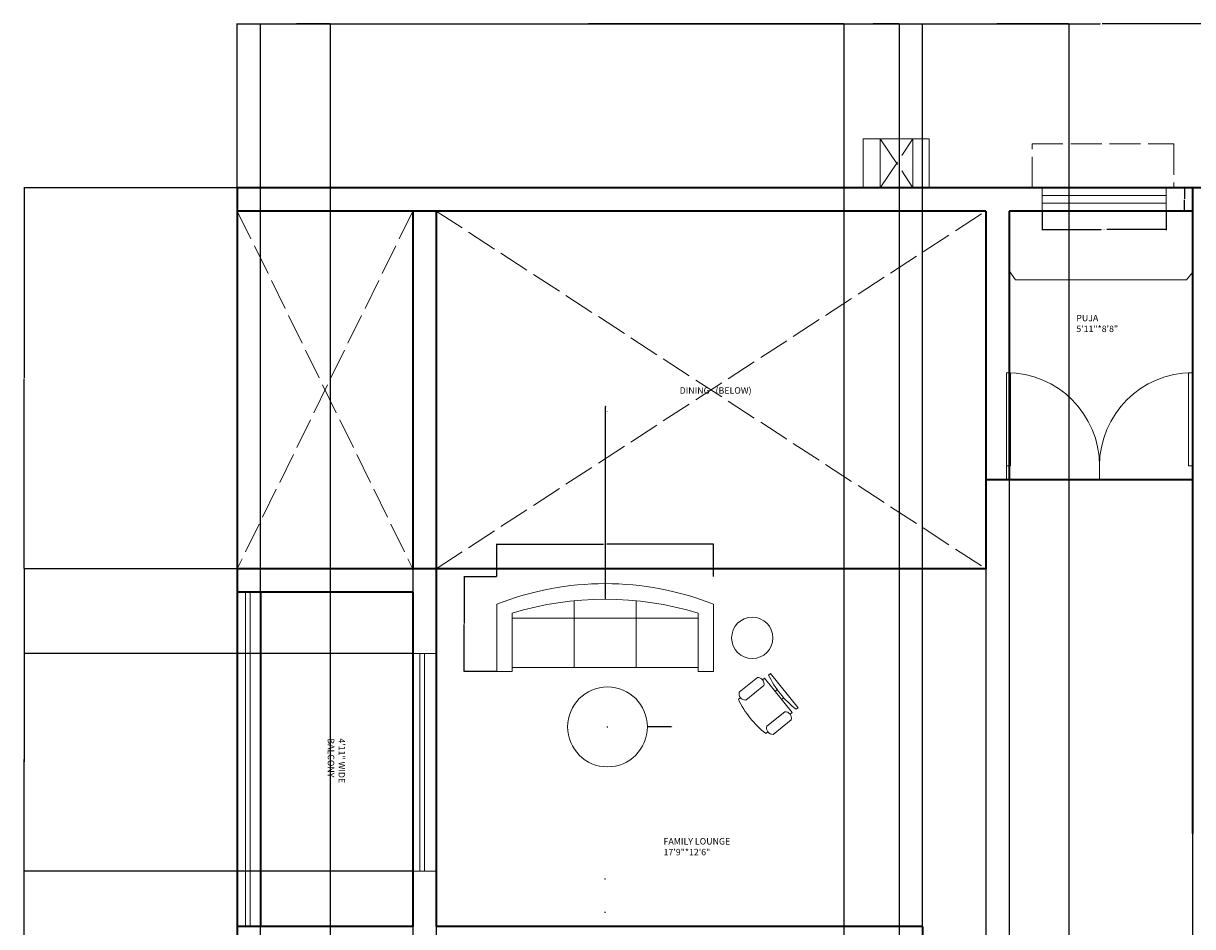
# Model space of a CAD drawing. Units: inches. Extents: x 293720 to 590083, y 155482 to 312405.
# Tile 3 of 4: x 293720 to 294173, y 156028 to 156378. Entities that reach past the tile are written whole.
import ezdxf

# ---------------------------------------------------------------- set-up
doc = ezdxf.new("R2010")
doc.units = ezdxf.units.IN
doc.linetypes.add('ACAD_ISO02W100', pattern=[15, 12, -3])
for name, color, linetype, lineweight in [('A-ANNO-DIMS', 2, 'Continuous', 18), ('A-AREA-IDEN', 7, 'Continuous', 18), ('A-DOOR', 3, 'Continuous', 18), ('A-FLOR-CASE', 8, 'Continuous', 18), ('A-FLOR-HRAL', 4, 'Continuous', 18), ('A-FLOR-OPEN', 8, 'ACAD_ISO02W100', 13), ('A-FLOR-OVHD', 8, 'ACAD_ISO02W100', 13), ('A-FLOR-PROJ', 8, 'Continuous', 18), ('A-FURN', 8, 'Continuous', 18), ('A-GLAZ', 4, 'Continuous', 18), ('A-WALL', 7, 'Continuous', 35)]:
    doc.layers.add(name, color=color, linetype=linetype, lineweight=lineweight)
doc.styles.get("Standard").update_dxf_attribs({"font": 'arial.ttf'})
doc.dimstyles.get("Standard").update_dxf_attribs({"dimtxt": 0.18, "dimasz": 0.18, "dimexe": 0.18, "dimexo": 0.0625, "dimgap": 0.09, "dimtad": 0, "dimtih": 1, "dimtoh": 1, "dimdec": 4, "dimzin": 0, "dimdsep": 46, "dimtxsty": 'Standard', "dimcen": 0.09, "dimadec": 0, "dimazin": 0, "dimtfac": 1, "dimtdec": 4, "dimtofl": 0, "dimtmove": 0, "dimatfit": 3, "dimfxl": 1, "dimtolj": 1, "dimtzin": 0, "dimarcsym": 0})

# ---------------------------------------------------------------- blocks, each defined once
blk = doc.blocks.new('Sofa - Roundback 7 ft.')
for p, q in [((-12.00002, -32.4421), (-12.00003, -6.5971)), ((11.99997, -32.4421), (11.99998, -6.5971)), ((-36.000027, -34), (-36.000027, -11.4696)), ((-35.999844, -13.3819), (35.9998, -13.3819)), ((35.99998, -34), (35.99998, -11.4696)), ((-36.000027, -32.4421), (35.99998, -32.4421))]:
    blk.add_line(p, q)
for points in [[(-36.000027, -34), (-42.000027, -34), (-42.000027, -8)], [(41.99998, -8), (41.99998, -34), (35.99998, -34)]]:
    blk.add_lwpolyline(points)
for centre, radius, start, end in [((0, -114.25), 114.25, 68.43141, 111.5686), ((-0.00001, -127.1968), 121.1968, 72.72033, 107.2797)]:
    blk.add_arc(centre, radius, start, end)
blk = doc.blocks.new('Chair - Desk')
for p, q in [((-8.5, 0), (-8.5, -1)), ((-8.5, 0), (8.5, 0)), ((8.5, 0), (8.5, -1)), ((-8.5, -3), (-8.5, -4)), ((-8.5, -3), (8.5, -3)), ((-2, -3), (-2, -1.9355)), ((2, -1.9576), (2, -3)), ((8.5, -3), (8.5, -4)), ((-10.5, -5), (-10.5, -14)), ((-6.5, -14), (-6.5, -5)), ((6.5, -5), (6.5, -14)), ((10.5, -14), (10.5, -5)), ((-8.5, -15), (-8.5, -16)), ((8.5, -15), (8.5, -16))]:
    blk.add_line(p, q)
for centre, radius, start, end in [((-8.5, -6.5), 2.5, 36.8699, 143.1301), ((0, 34.625), 36.625, 256.5803, 283.4197), ((8.5, -6.5), 2.5, 36.8699, 143.1301), ((-8.5, -12.5), 2.5, 216.8699, 323.1301), ((0, 19.625), 36.625, 256.5803, 283.4197), ((8.5, -12.5), 2.5, 216.8699, 323.1301)]:
    blk.add_arc(centre, radius, start, end)
blk = doc.blocks.new('*U2')
for p, q in [((0, 0), (0, -6)), ((40, 0), (40, -6))]:
    blk.add_line(p, q)
blk.add_lwpolyline([(0, 0), (0, 40), (1.75, 40), (1.75, 0)], close=True)
blk.add_arc((0, 0), 40, 0, 90)
blk = doc.blocks.new('WIN-48IN')
for p, q in [((0, 9), (48, 9)), ((0, 0), (0, 9)), ((0, 6), (48, 6)), ((48, 9), (48, 0)), ((48, 3), (0, 3)), ((48, 0), (0, 0))]:
    blk.add_line(p, q)
blk = doc.blocks.new('*D37')
at = {"layer": 'A-ANNO-DIMS', "color": 0, "lineweight": -2, "transparency": 16777216}
for p, q in [((294114.85, 156304.87), (294114.85, 156297.55)), ((294162.85, 156304.87), (294162.85, 156297.55)), ((294115.03, 156297.73), (294137.73, 156297.73)), ((294162.67, 156297.73), (294139.96, 156297.73))]:
    blk.add_line(p, q, dxfattribs=at)
at = {"layer": 'A-ANNO-DIMS', "color": 0, "lineweight": 100, "transparency": 16777216}
for points in [[(294115.03, 156297.76), (294115.03, 156297.7), (294114.85, 156297.73)], [(294162.67, 156297.76), (294162.67, 156297.7), (294162.85, 156297.73)]]:
    blk.add_solid(points, dxfattribs=at)
at = {"layer": 'Defpoints', "color": 0, "lineweight": 100, "transparency": 16777216}
for p in [(294114.85, 156304.93), (294162.85, 156304.93), (294162.85, 156297.73)]:
    blk.add_point(p, dxfattribs=at)
at = {"layer": 'A-ANNO-DIMS', "color": 0, "transparency": 16777216, "insert": (294138.85, 156297.73), "char_height": 0.18, "attachment_point": 5}
blk.add_mtext('\\A1;WINDOW 48 TYP.', dxfattribs=at)
blk = doc.blocks.new('*D38')
at = {"layer": 'A-ANNO-DIMS', "color": 0, "lineweight": -2, "transparency": 16777216}
for p, q in [((294162.91, 156313.93), (294170.23, 156313.93)), ((294170.05, 156313.75), (294170.05, 156309.61)), ((294170.05, 156305.11), (294170.05, 156309.25)), ((294162.91, 156304.93), (294170.23, 156304.93))]:
    blk.add_line(p, q, dxfattribs=at)
at = {"layer": 'A-ANNO-DIMS', "color": 0, "lineweight": 100, "transparency": 16777216}
for points in [[(294170.02, 156313.75), (294170.08, 156313.75), (294170.05, 156313.93)], [(294170.02, 156305.11), (294170.08, 156305.11), (294170.05, 156304.93)]]:
    blk.add_solid(points, dxfattribs=at)
at = {"layer": 'Defpoints', "color": 0, "lineweight": 100, "transparency": 16777216}
for p in [(294162.85, 156313.93), (294170.05, 156313.93), (294162.85, 156304.93)]:
    blk.add_point(p, dxfattribs=at)
at = {"layer": 'A-ANNO-DIMS', "color": 0, "transparency": 16777216, "insert": (294170.05, 156309.43), "char_height": 0.18, "attachment_point": 5}
blk.add_mtext('\\A1;9 TYP.', dxfattribs=at)
blk = doc.blocks.new('*D51')
at = {"layer": 'A-ANNO-DIMS', "color": 0, "lineweight": -2, "transparency": 16777216}
for p, q in [((293903.6, 156163.42), (293903.6, 156176.14)), ((293903.78, 156175.96), (293945, 156175.96)), ((293987.42, 156175.96), (293946.19, 156175.96)), ((293987.6, 156163.42), (293987.6, 156176.14))]:
    blk.add_line(p, q, dxfattribs=at)
at = {"layer": 'A-ANNO-DIMS', "color": 0, "lineweight": 100, "transparency": 16777216}
for points in [[(293903.78, 156175.99), (293903.78, 156175.93), (293903.6, 156175.96)], [(293987.42, 156175.99), (293987.42, 156175.93), (293987.6, 156175.96)]]:
    blk.add_solid(points, dxfattribs=at)
at = {"layer": 'Defpoints', "color": 0, "lineweight": 100, "transparency": 16777216}
for p in [(293987.6, 156175.96), (293903.6, 156163.36), (293987.6, 156163.36)]:
    blk.add_point(p, dxfattribs=at)
at = {"layer": 'A-ANNO-DIMS', "color": 0, "transparency": 16777216, "insert": (293945.6, 156175.96), "char_height": 0.18, "attachment_point": 5}
blk.add_mtext('\\A1;SOFA 84', dxfattribs=at)
blk = doc.blocks.new('*D52')
at = {"layer": 'A-ANNO-DIMS', "color": 0, "lineweight": -2, "transparency": 16777216}
for p, q in [((293903.54, 156163.36), (293890.82, 156163.36)), ((293891, 156163.18), (293891, 156145.21)), ((293891, 156126.87), (293891, 156144.84)), ((293903.54, 156126.69), (293890.82, 156126.69))]:
    blk.add_line(p, q, dxfattribs=at)
at = {"layer": 'A-ANNO-DIMS', "color": 0, "lineweight": 100, "transparency": 16777216}
for points in [[(293890.97, 156163.18), (293891.03, 156163.18), (293891, 156163.36)], [(293890.97, 156126.87), (293891.03, 156126.87), (293891, 156126.69)]]:
    blk.add_solid(points, dxfattribs=at)
at = {"layer": 'Defpoints', "color": 0, "lineweight": 100, "transparency": 16777216}
for p in [(293891, 156163.36), (293903.6, 156163.36), (293903.6, 156126.69)]:
    blk.add_point(p, dxfattribs=at)
at = {"layer": 'A-ANNO-DIMS', "color": 0, "transparency": 16777216, "insert": (293891, 156145.03), "char_height": 0.18, "attachment_point": 5}
blk.add_mtext('\\A1;37', dxfattribs=at)
blk = doc.blocks.new('*D53')
at = {"layer": 'A-ANNO-DIMS', "color": 0, "lineweight": -2, "transparency": 16777216}
for p, q in [((294499.07, 156062.55), (294499.07, 155481.85)), ((293762.89, 155594.88), (293762.89, 155481.85)), ((293763.07, 155482.03), (294130.59, 155482.03)), ((294498.89, 155482.03), (294131.37, 155482.03))]:
    blk.add_line(p, q, dxfattribs=at)
at = {"layer": 'A-ANNO-DIMS', "color": 0, "lineweight": 100, "transparency": 16777216}
for points in [[(293763.07, 155482.06), (293763.07, 155482), (293762.89, 155482.03)], [(294498.89, 155482.06), (294498.89, 155482), (294499.07, 155482.03)]]:
    blk.add_solid(points, dxfattribs=at)
at = {"layer": 'Defpoints', "color": 0, "lineweight": 100, "transparency": 16777216}
for p in [(294499.07, 156062.61), (293762.89, 155594.94), (294499.07, 155482.03)]:
    blk.add_point(p, dxfattribs=at)
at = {"layer": 'A-ANNO-DIMS', "color": 0, "transparency": 16777216, "insert": (294130.98, 155482.03), "char_height": 0.18, "attachment_point": 5}
blk.add_mtext('\\A1;736.2', dxfattribs=at)
blk = doc.blocks.new('*D55')
at = {"layer": 'A-ANNO-DIMS', "color": 0, "lineweight": -2, "transparency": 16777216}
for p, q in [((293803.09, 156313.99), (293803.09, 156377.57)), ((293803.27, 156377.39), (294137.29, 156377.39)), ((294472.1, 156377.39), (294138.08, 156377.39)), ((294472.28, 156335.1), (294472.28, 156377.57))]:
    blk.add_line(p, q, dxfattribs=at)
at = {"layer": 'A-ANNO-DIMS', "color": 0, "lineweight": 100, "transparency": 16777216}
for points in [[(293803.27, 156377.42), (293803.27, 156377.36), (293803.09, 156377.39)], [(294472.1, 156377.42), (294472.1, 156377.36), (294472.28, 156377.39)]]:
    blk.add_solid(points, dxfattribs=at)
at = {"layer": 'Defpoints', "color": 0, "lineweight": 100, "transparency": 16777216}
for p in [(294472.28, 156377.39), (294472.28, 156335.04), (293803.09, 156313.93)]:
    blk.add_point(p, dxfattribs=at)
at = {"layer": 'A-ANNO-DIMS', "color": 0, "transparency": 16777216, "insert": (294137.68, 156377.39), "char_height": 0.18, "attachment_point": 5}
blk.add_mtext('\\A1;669.2', dxfattribs=at)
blk = doc.blocks.new('*D56')
at = {"layer": 'A-ANNO-DIMS', "color": 0, "lineweight": -2, "transparency": 16777216}
for p, q in [((293803.09, 156304.87), (293803.09, 155481.85)), ((293871.09, 156304.87), (293871.09, 155481.85)), ((293803.27, 155482.03), (293836.87, 155482.03)), ((293870.91, 155482.03), (293837.31, 155482.03))]:
    blk.add_line(p, q, dxfattribs=at)
at = {"layer": 'A-ANNO-DIMS', "color": 0, "lineweight": 100, "transparency": 16777216}
for points in [[(293803.27, 155482.06), (293803.27, 155482), (293803.09, 155482.03)], [(293870.91, 155482.06), (293870.91, 155482), (293871.09, 155482.03)]]:
    blk.add_solid(points, dxfattribs=at)
at = {"layer": 'Defpoints', "color": 0, "lineweight": 100, "transparency": 16777216}
for p in [(293803.09, 156304.93), (293871.09, 156304.93), (293871.09, 155482.03)]:
    blk.add_point(p, dxfattribs=at)
at = {"layer": 'A-ANNO-DIMS', "color": 0, "transparency": 16777216, "insert": (293837.09, 155482.03), "char_height": 0.18, "attachment_point": 5}
blk.add_mtext('\\A1;68', dxfattribs=at)
blk = doc.blocks.new('*D57')
at = {"layer": 'A-ANNO-DIMS', "color": 0, "lineweight": -2, "transparency": 16777216}
for p, q in [((293880.093104, 156304.865707), (293880.093104, 155481.8534)), ((294093.093104, 156304.865707), (294093.093104, 155481.8534)), ((293880.273104, 155482.0334), (293986.302722, 155482.0334)), ((294092.913104, 155482.0334), (293986.883486, 155482.0334))]:
    blk.add_line(p, q, dxfattribs=at)
at = {"layer": 'A-ANNO-DIMS', "color": 0, "lineweight": 100, "transparency": 16777216}
for points in [[(293880.273104, 155482.0634), (293880.273104, 155482.0034), (293880.093104, 155482.0334)], [(294092.913104, 155482.0634), (294092.913104, 155482.0034), (294093.093104, 155482.0334)]]:
    blk.add_solid(points, dxfattribs=at)
at = {"layer": 'Defpoints', "color": 0, "lineweight": 100, "transparency": 16777216}
for p in [(293880.093104, 156304.928207), (294093.093104, 156304.928207), (294093.093104, 155482.0334)]:
    blk.add_point(p, dxfattribs=at)
at = {"layer": 'A-ANNO-DIMS', "color": 0, "transparency": 16777216, "insert": (293986.593104, 155482.0334), "char_height": 0.18, "attachment_point": 5}
blk.add_mtext('\\A1;213', dxfattribs=at)
blk = doc.blocks.new('*D58')
at = {"layer": 'A-ANNO-DIMS', "color": 0, "lineweight": -2, "transparency": 16777216}
for p, q in [((294102.09, 156200.87), (294102.09, 155481.85)), ((294173.09, 156200.87), (294173.09, 155481.85)), ((294102.27, 155482.03), (294137.39, 155482.03)), ((294172.91, 155482.03), (294137.79, 155482.03))]:
    blk.add_line(p, q, dxfattribs=at)
at = {"layer": 'A-ANNO-DIMS', "color": 0, "lineweight": 100, "transparency": 16777216}
for points in [[(294102.27, 155482.06), (294102.27, 155482), (294102.09, 155482.03)], [(294172.91, 155482.06), (294172.91, 155482), (294173.09, 155482.03)]]:
    blk.add_solid(points, dxfattribs=at)
at = {"layer": 'Defpoints', "color": 0, "lineweight": 100, "transparency": 16777216}
for p in [(294102.09, 156200.93), (294173.09, 156200.93), (294173.09, 155482.03)]:
    blk.add_point(p, dxfattribs=at)
at = {"layer": 'A-ANNO-DIMS', "color": 0, "transparency": 16777216, "insert": (294137.59, 155482.03), "char_height": 0.18, "attachment_point": 5}
blk.add_mtext('\\A1;71', dxfattribs=at)
blk = doc.blocks.new('*D64')
at = {"layer": 'A-ANNO-DIMS', "color": 0, "lineweight": -2, "transparency": 16777216}
for p, q in [((293803.03, 156166.43), (293720.36, 156166.43)), ((293720.54, 156166.25), (293720.54, 156092.86)), ((293720.54, 156019.11), (293720.54, 156092.5)), ((293812.03, 156018.93), (293720.36, 156018.93))]:
    blk.add_line(p, q, dxfattribs=at)
at = {"layer": 'A-ANNO-DIMS', "color": 0, "lineweight": 100, "transparency": 16777216}
for points in [[(293720.51, 156166.25), (293720.57, 156166.25), (293720.54, 156166.43)], [(293720.51, 156019.11), (293720.57, 156019.11), (293720.54, 156018.93)]]:
    blk.add_solid(points, dxfattribs=at)
at = {"layer": 'Defpoints', "color": 0, "lineweight": 100, "transparency": 16777216}
for p in [(293720.54, 156166.43), (293803.09, 156166.43), (293812.09, 156018.93)]:
    blk.add_point(p, dxfattribs=at)
at = {"layer": 'A-ANNO-DIMS', "color": 0, "transparency": 16777216, "insert": (293720.54, 156092.68), "char_height": 0.18, "attachment_point": 5}
blk.add_mtext('\\A1;147.5', dxfattribs=at)
blk = doc.blocks.new('*D65')
at = {"layer": 'A-ANNO-DIMS', "color": 0, "lineweight": -2, "transparency": 16777216}
for p, q in [((293803.03, 156313.93), (293720.36, 156313.93)), ((293720.54, 156313.75), (293720.54, 156240.36)), ((293720.54, 156166.61), (293720.54, 156240)), ((293803.03, 156166.43), (293720.36, 156166.43))]:
    blk.add_line(p, q, dxfattribs=at)
at = {"layer": 'A-ANNO-DIMS', "color": 0, "lineweight": 100, "transparency": 16777216}
for points in [[(293720.51, 156313.75), (293720.57, 156313.75), (293720.54, 156313.93)], [(293720.51, 156166.61), (293720.57, 156166.61), (293720.54, 156166.43)]]:
    blk.add_solid(points, dxfattribs=at)
at = {"layer": 'Defpoints', "color": 0, "lineweight": 100, "transparency": 16777216}
for p in [(293720.54, 156313.93), (293803.09, 156313.93), (293803.09, 156166.43)]:
    blk.add_point(p, dxfattribs=at)
at = {"layer": 'A-ANNO-DIMS', "color": 0, "transparency": 16777216, "insert": (293720.54, 156240.18), "char_height": 0.18, "attachment_point": 5}
blk.add_mtext('\\A1;147.5', dxfattribs=at)
blk = doc.blocks.new('*D66')
at = {"layer": 'A-ANNO-DIMS', "color": 0, "lineweight": -2, "transparency": 16777216}
for p, q in [((293812.09, 155556.99), (293812.09, 156377.57)), ((293812.27, 156377.39), (293825.26, 156377.39)), ((293839.03, 156377.39), (293826.05, 156377.39)), ((293839.21, 155556.99), (293839.21, 156377.57))]:
    blk.add_line(p, q, dxfattribs=at)
at = {"layer": 'A-ANNO-DIMS', "color": 0, "lineweight": 100, "transparency": 16777216}
for points in [[(293812.27, 156377.42), (293812.27, 156377.36), (293812.09, 156377.39)], [(293839.03, 156377.42), (293839.03, 156377.36), (293839.21, 156377.39)]]:
    blk.add_solid(points, dxfattribs=at)
at = {"layer": 'Defpoints', "color": 0, "lineweight": 100, "transparency": 16777216}
for p in [(293839.21, 156377.39), (293812.09, 155556.93), (293839.21, 155556.93)]:
    blk.add_point(p, dxfattribs=at)
at = {"layer": 'A-ANNO-DIMS', "color": 0, "transparency": 16777216, "insert": (293825.65, 156377.39), "char_height": 0.18, "attachment_point": 5}
blk.add_mtext('\\A1;27.12', dxfattribs=at)
blk = doc.blocks.new('*D67')
at = {"layer": 'A-ANNO-DIMS', "color": 0, "lineweight": -2, "transparency": 16777216}
for p, q in [((293839.21, 155556.99), (293839.21, 156377.57)), ((293839.39, 156377.39), (293938.24, 156377.39)), ((294038, 156377.39), (293939.15, 156377.39)), ((294038.18, 155556.99), (294038.18, 156377.57))]:
    blk.add_line(p, q, dxfattribs=at)
at = {"layer": 'A-ANNO-DIMS', "color": 0, "lineweight": 100, "transparency": 16777216}
for points in [[(293839.39, 156377.42), (293839.39, 156377.36), (293839.21, 156377.39)], [(294038, 156377.42), (294038, 156377.36), (294038.18, 156377.39)]]:
    blk.add_solid(points, dxfattribs=at)
at = {"layer": 'Defpoints', "color": 0, "lineweight": 100, "transparency": 16777216}
for p in [(294038.18, 156377.39), (293839.21, 155556.93), (294038.18, 155556.93)]:
    blk.add_point(p, dxfattribs=at)
at = {"layer": 'A-ANNO-DIMS', "color": 0, "transparency": 16777216, "insert": (293938.7, 156377.39), "char_height": 0.18, "attachment_point": 5}
blk.add_mtext('\\A1;198.97', dxfattribs=at)
blk = doc.blocks.new('*D68')
at = {"layer": 'A-ANNO-DIMS', "color": 0, "lineweight": -2, "transparency": 16777216}
for p, q in [((294038.180795, 155556.990707), (294038.180795, 156377.567612)), ((294038.360795, 156377.387612), (294048.417601, 156377.387612)), ((294059.406085, 156377.387612), (294049.349279, 156377.387612)), ((294059.586085, 155556.990707), (294059.586085, 156377.567612))]:
    blk.add_line(p, q, dxfattribs=at)
at = {"layer": 'A-ANNO-DIMS', "color": 0, "lineweight": 100, "transparency": 16777216}
for points in [[(294038.360795, 156377.417612), (294038.360795, 156377.357612), (294038.180795, 156377.387612)], [(294059.406085, 156377.417612), (294059.406085, 156377.357612), (294059.586085, 156377.387612)]]:
    blk.add_solid(points, dxfattribs=at)
at = {"layer": 'Defpoints', "color": 0, "lineweight": 100, "transparency": 16777216}
for p in [(294059.586085, 156377.387612), (294038.180795, 155556.928207), (294059.586085, 155556.928207)]:
    blk.add_point(p, dxfattribs=at)
at = {"layer": 'A-ANNO-DIMS', "color": 0, "transparency": 16777216, "insert": (294048.88344, 156377.387612), "char_height": 0.18, "attachment_point": 5}
blk.add_mtext('\\A1;21.405', dxfattribs=at)
blk = doc.blocks.new('*D69')
at = {"layer": 'A-ANNO-DIMS', "color": 0, "lineweight": -2, "transparency": 16777216}
for p, q in [((294068.586085, 155556.990707), (294068.586085, 156377.567612)), ((294068.766085, 156377.387612), (294096.611145, 156377.387612)), ((294125.103763, 156377.387612), (294097.258703, 156377.387612)), ((294125.283763, 155556.990707), (294125.283763, 156377.567612))]:
    blk.add_line(p, q, dxfattribs=at)
at = {"layer": 'A-ANNO-DIMS', "color": 0, "lineweight": 100, "transparency": 16777216}
for points in [[(294068.766085, 156377.417612), (294068.766085, 156377.357612), (294068.586085, 156377.387612)], [(294125.103763, 156377.417612), (294125.103763, 156377.357612), (294125.283763, 156377.387612)]]:
    blk.add_solid(points, dxfattribs=at)
at = {"layer": 'Defpoints', "color": 0, "lineweight": 100, "transparency": 16777216}
for p in [(294125.283763, 156377.387612), (294068.586085, 155556.928207), (294125.283763, 155556.928207)]:
    blk.add_point(p, dxfattribs=at)
at = {"layer": 'A-ANNO-DIMS', "color": 0, "transparency": 16777216, "insert": (294096.934924, 156377.387612), "char_height": 0.18, "attachment_point": 5}
blk.add_mtext('\\A1;56.7', dxfattribs=at)
blk = doc.blocks.new('*D74')
at = {"layer": 'A-ANNO-DIMS', "color": 0, "lineweight": -2, "transparency": 16777216}
for p, q in [((293871.03, 156133.66), (293720.36, 156133.66)), ((293720.54, 156133.48), (293720.54, 156091.69)), ((293720.54, 156049.53), (293720.54, 156091.32)), ((293871.03, 156049.35), (293720.36, 156049.35))]:
    blk.add_line(p, q, dxfattribs=at)
at = {"layer": 'A-ANNO-DIMS', "color": 0, "lineweight": 100, "transparency": 16777216}
for points in [[(293720.51, 156133.48), (293720.57, 156133.48), (293720.54, 156133.66)], [(293720.51, 156049.53), (293720.57, 156049.53), (293720.54, 156049.35)]]:
    blk.add_solid(points, dxfattribs=at)
at = {"layer": 'Defpoints', "color": 0, "lineweight": 100, "transparency": 16777216}
for p in [(293720.54, 156133.66), (293871.09, 156133.66), (293871.09, 156049.35)]:
    blk.add_point(p, dxfattribs=at)
at = {"layer": 'A-ANNO-DIMS', "color": 0, "transparency": 16777216, "insert": (293720.54, 156091.5), "char_height": 0.18, "attachment_point": 5}
blk.add_mtext('\\A1;84.3', dxfattribs=at)
blk = doc.blocks.new('*D77')
at = {"layer": 'A-ANNO-DIMS', "color": 0, "lineweight": -2, "transparency": 16777216}
for p, q in [((293946.41, 156105.24), (293946.59, 156105.24)), ((293946.5, 156105.15), (293946.5, 156105.33)), ((293971.24, 156105.24), (293962.14, 156105.24))]:
    blk.add_line(p, q, dxfattribs=at)
at = {"layer": 'A-ANNO-DIMS', "color": 0, "lineweight": 100, "transparency": 16777216}
blk.add_solid([(293962.14, 156105.27), (293962.14, 156105.21), (293961.96, 156105.24)], dxfattribs=at)
at = {"layer": 'Defpoints', "color": 0, "lineweight": 100, "transparency": 16777216}
for p in [(293931.03, 156105.24), (293961.96, 156105.24)]:
    blk.add_point(p, dxfattribs=at)
at = {"layer": 'A-ANNO-DIMS', "color": 0, "transparency": 16777216, "insert": (293971.74, 156105.24), "char_height": 0.18, "attachment_point": 5}
blk.add_mtext('\\A1;∅30.93', dxfattribs=at)
blk = doc.blocks.new('*D79')
at = {"layer": 'A-ANNO-DIMS', "color": 0, "lineweight": -2, "transparency": 16777216}
for p, q in [((293945.78, 156227.41), (293945.6, 156227.41)), ((293945.6, 156227.41), (293945.6, 156154.87)), ((293945.51, 156033.49), (293945.69, 156033.49)), ((293945.6, 156033.4), (293945.6, 156033.58))]:
    blk.add_line(p, q, dxfattribs=at)
at = {"layer": 'A-ANNO-DIMS', "color": 0, "lineweight": 100, "transparency": 16777216}
blk.add_solid([(293945.57, 156154.87), (293945.63, 156154.87), (293945.6, 156154.69)], dxfattribs=at)
at = {"layer": 'Defpoints', "color": 0, "lineweight": 100, "transparency": 16777216}
for p in [(293945.6, 156154.69), (293945.6, 156033.49)]:
    blk.add_point(p, dxfattribs=at)
at = {"layer": 'A-ANNO-DIMS', "color": 0, "transparency": 16777216, "insert": (293946.26, 156227.41), "char_height": 0.18, "attachment_point": 5}
blk.add_mtext('\\A1;R121.2', dxfattribs=at)
blk = doc.blocks.new('*D80')
at = {"layer": 'A-ANNO-DIMS', "color": 0, "lineweight": -2, "transparency": 16777216}
for p, q in [((293945.78, 156229.24), (293945.6, 156229.24)), ((293945.6, 156229.24), (293945.6, 156160.87)), ((293945.51, 156046.44), (293945.69, 156046.44)), ((293945.6, 156046.35), (293945.6, 156046.53))]:
    blk.add_line(p, q, dxfattribs=at)
at = {"layer": 'A-ANNO-DIMS', "color": 0, "lineweight": 100, "transparency": 16777216}
blk.add_solid([(293945.57, 156160.87), (293945.63, 156160.87), (293945.6, 156160.69)], dxfattribs=at)
at = {"layer": 'Defpoints', "color": 0, "lineweight": 100, "transparency": 16777216}
for p in [(293945.6, 156160.69), (293945.6, 156046.44)]:
    blk.add_point(p, dxfattribs=at)
at = {"layer": 'A-ANNO-DIMS', "color": 0, "transparency": 16777216, "insert": (293946.33, 156229.24), "char_height": 0.18, "attachment_point": 5}
blk.add_mtext('\\A1;R114.25', dxfattribs=at)

msp = doc.modelspace()

# ---------------------------------------------------------------- linework, layer by layer
at = {"layer": 'A-FLOR-CASE'}
for p, q in [((294104.5389, 156278.236), (294102.0931, 156281.772)), ((294170.8462, 156278.236), (294104.5389, 156278.236)), ((294170.8462, 156278.236), (294173.0931, 156281.1725))]:
    msp.add_line(p, q, dxfattribs=at)
at = {"layer": 'A-FLOR-HRAL'}
for p, q in [((293806.2773, 156157.2673), (293806.2773, 156027.9282)), ((293808.1204, 156157.4282), (293808.1204, 156027.9282))]:
    msp.add_line(p, q, dxfattribs=at)
at = {"layer": 'A-FLOR-OPEN'}
for p, q in [((294052.1148, 156332.9027), (294064.8378, 156313.9282)), ((294052.1148, 156313.9282), (294064.8378, 156332.9027)), ((293871.0931, 156304.9282), (293803.0931, 156166.4282)), ((293803.0931, 156304.9282), (293871.0931, 156166.4282)), ((293880.0931, 156304.9282), (294093.0931, 156166.4282)), ((293880.0931, 156166.4282), (294093.0931, 156304.9282))]:
    msp.add_line(p, q, dxfattribs=at)
at = {"layer": 'A-FLOR-OVHD'}
for p, q in [((294110.9417, 156313.9282), (294110.9417, 156330.9221)), ((294110.9417, 156330.9221), (294165.8377, 156330.9221)), ((294165.8377, 156330.9221), (294165.8377, 156313.9282))]:
    msp.add_line(p, q, dxfattribs=at)
at = {"layer": 'A-FLOR-PROJ'}
for p, q in [((294052.1148, 156332.9027), (294045.5867, 156332.9027)), ((294045.5867, 156332.9027), (294045.5867, 156313.9282)), ((294064.8378, 156332.9027), (294052.1148, 156332.9027)), ((294052.1148, 156332.9027), (294052.1148, 156313.9282)), ((294071.067, 156332.9027), (294064.8378, 156332.9027)), ((294064.8378, 156332.9027), (294064.8378, 156313.9282)), ((294071.067, 156313.9282), (294071.067, 156332.9027))]:
    msp.add_line(p, q, dxfattribs=at)
at = {"layer": 'A-FURN'}
for centre, radius in [((294002.5787, 156139.6981), 8.0069), ((293946.4984, 156105.2361), 15.4658)]:
    msp.add_circle(centre, radius, dxfattribs=at)
at = {"layer": 'A-GLAZ'}
for p, q in [((293871.0931, 156133.6571), (293880.0931, 156133.6571)), ((293873.824, 156133.6571), (293873.824, 156049.3526)), ((293875.5931, 156133.6571), (293875.5931, 156049.3526)), ((293871.0931, 156049.3526), (293880.0931, 156049.3526))]:
    msp.add_line(p, q, dxfattribs=at)
at = {"layer": 'A-WALL'}
for p, q in [((294412.0931, 156313.9282), (293803.0931, 156313.9282)), ((293803.0931, 156313.9282), (293803.0931, 155547.9282)), ((294173.0931, 156313.9282), (294173.0931, 156070.5313)), ((293880.0931, 156304.9282), (293803.0931, 156304.9282)), ((293871.0931, 156304.9282), (293871.0931, 156166.4282)), ((293880.0931, 156304.9282), (293880.0931, 156027.9282)), ((294093.0931, 156304.9282), (293880.0931, 156304.9282)), ((294093.0931, 156304.9282), (294093.0931, 156166.4282)), ((294102.0931, 156304.9282), (294102.0931, 156200.9282)), ((294173.0931, 156304.9282), (294102.0931, 156304.9282)), ((294173.0931, 156200.9282), (294093.0931, 156200.9282)), ((294093.0931, 156166.4282), (293803.0931, 156166.4282)), ((293871.0931, 156157.4282), (293803.0931, 156157.4282)), ((293812.0931, 156157.4282), (293812.0931, 156027.9282)), ((293871.0931, 156157.4282), (293871.0931, 156027.9282)), ((294173.0931, 156070.5313), (294173.1558, 156063.9282)), ((293871.0931, 156027.9282), (293803.0931, 156027.9282)), ((294068.5861, 156027.9282), (293880.0931, 156027.9282)), ((294068.5861, 156018.9282), (294068.5861, 156027.9282))]:
    msp.add_line(p, q, dxfattribs=at)

# ---------------------------------------------------------------- block references
at = {"layer": 'A-DOOR', "yscale": 0.9, "zscale": 0.9}
for p, xscale in [((294101.0931, 156206.3514), 0.9), ((294173.0931, 156206.3282), -0.9)]:
    msp.add_blockref('*U2', p, dxfattribs=dict(at, xscale=xscale))
at = {"layer": 'A-FURN'}
msp.add_blockref('Sofa - Roundback 7 ft.', (293945.5977, 156160.6917), dxfattribs=at)
at = {"layer": 'A-FURN', "rotation": 308.7351697626769}
msp.add_blockref('Chair - Desk', (294015.0194, 156119.302), dxfattribs=at)
at = {"layer": 'A-GLAZ'}
msp.add_blockref('WIN-48IN', (294114.846, 156304.928), dxfattribs=at)

# ---------------------------------------------------------------- texts
at = {"layer": 'A-AREA-IDEN', "char_height": 2.5, "attachment_point": 1}
for s, width, insert in [('PUJA\\P5\'11"*8\'8"', 37.416236, (294128.1037, 156264.7418)), ('DINING   (BELOW)', 112.755918, (293974.4439, 156236.7193)), ('FAMILY LOUNGE\\P17\'9"*12\'6"', 95.76668, (293968.216, 156062.1883))]:
    msp.add_mtext_dynamic_manual_height_columns(s, width=width, gutter_width=12.5, heights=[0], dxfattribs=dict(at, insert=insert))
at = {"layer": 'A-AREA-IDEN', "insert": (293844.8114, 156100.8087), "char_height": 2.5, "attachment_point": 1, "rotation": 270}
msp.add_mtext_dynamic_manual_height_columns('4\'11" WIDE \\PBALCONY', width=38.193219, gutter_width=12.5, heights=[0], dxfattribs=at)

# ---------------------------------------------------------------- dimensions: what is measured, and where the dimension line sits
at = {"layer": 'A-ANNO-DIMS'}
for base, p1, p2, override, picture, middle in [((294472.2763, 156377.3876), (293803.0931, 156313.9282), (294472.2763, 156335.0376), {"dimdec": 1, "dimlfac": 1, "dimrnd": 0, "dimzin": 0, "dimdsep": 46, "dimlunit": 2}, '*D55', (294137.6847, 156377.3876)), ((293839.2106, 156377.3876), (293812.0931, 155556.9282), (293839.2106, 155556.9282), {"dimdec": 2, "dimlfac": 1, "dimrnd": 0, "dimzin": 0, "dimdsep": 46, "dimlunit": 2}, '*D66', (293825.6519, 156377.3876)), ((294038.1808, 156377.3876), (293839.2106, 155556.9282), (294038.1808, 155556.9282), {"dimdec": 2, "dimlfac": 1, "dimrnd": 0, "dimzin": 0, "dimdsep": 46, "dimlunit": 2}, '*D67', (293938.6957, 156377.3876)), ((294059.5861, 156377.3876), (294038.1808, 155556.9282), (294059.5861, 155556.9282), {"dimdec": 3, "dimlfac": 1, "dimrnd": 0, "dimzin": 0, "dimdsep": 46, "dimlunit": 2}, '*D68', (294048.8834, 156377.3876)), ((294125.2838, 156377.3876), (294068.5861, 155556.9282), (294125.2838, 155556.9282), {"dimdec": 1, "dimlfac": 1, "dimrnd": 0, "dimzin": 0, "dimdsep": 46, "dimlunit": 2}, '*D69', (294096.9349, 156377.3876)), ((293871.0931, 155482.0334), (293803.0931, 156304.9282), (293871.0931, 156304.9282), {"dimdec": 0, "dimlfac": 1, "dimrnd": 0, "dimzin": 0, "dimdsep": 46, "dimlunit": 2}, '*D56', (293837.0931, 155482.0334)), ((294093.0931, 155482.0334), (293880.0931, 156304.9282), (294093.0931, 156304.9282), {"dimdec": 0, "dimlfac": 1, "dimrnd": 0, "dimzin": 0, "dimdsep": 46, "dimlunit": 2}, '*D57', (293986.5931, 155482.0334)), ((294173.0931, 155482.0334), (294102.0931, 156200.9282), (294173.0931, 156200.9282), {"dimdec": 0, "dimlfac": 1, "dimrnd": 0, "dimzin": 0, "dimdsep": 46, "dimlunit": 2}, '*D58', (294137.5931, 155482.0334)), ((294499.0676, 155482.0334), (293762.8891, 155594.9386), (294499.0676, 156062.6102), {"dimdec": 1, "dimlfac": 1, "dimrnd": 0, "dimzin": 0, "dimdsep": 46, "dimlunit": 2}, '*D53', (294130.9783, 155482.0334))]:
    dim = msp.add_linear_dim(base=base, p1=p1, p2=p2, dimstyle='Standard', override=override, dxfattribs=at)
    dim.commit()
    dim.dimension.update_dxf_attribs({"geometry": picture, "text_midpoint": middle})
for base, p1, p2, override, picture, middle in [((293720.5391, 156313.9282), (293803.0931, 156166.4282), (293803.0931, 156313.9282), {"dimdec": 1, "dimlfac": 1, "dimrnd": 0, "dimzin": 0, "dimdsep": 46, "dimlunit": 2}, '*D65', (293720.5391, 156240.1782)), ((293720.5391, 156166.4282), (293812.0931, 156018.9282), (293803.0931, 156166.4282), {"dimdec": 1, "dimlfac": 1, "dimrnd": 0, "dimzin": 0, "dimdsep": 46, "dimlunit": 2}, '*D64', (293720.5391, 156092.6782)), ((293890.9977, 156163.3584), (293903.5977, 156126.6917), (293903.5977, 156163.3584), {"dimdec": 0, "dimlfac": 1, "dimrnd": 0, "dimzin": 0, "dimdsep": 46, "dimlunit": 2}, '*D52', (293890.9977, 156145.0251)), ((293720.5391, 156133.6571), (293871.0931, 156049.3526), (293871.0931, 156133.6571), {"dimdec": 1, "dimlfac": 1, "dimrnd": 0, "dimzin": 0, "dimdsep": 46, "dimlunit": 2}, '*D74', (293720.5391, 156091.5048))]:
    dim = msp.add_linear_dim(base=base, p1=p1, p2=p2, angle=90, dimstyle='Standard', override=override, dxfattribs=at)
    dim.commit()
    dim.dimension.update_dxf_attribs({"geometry": picture, "text_midpoint": middle})
dim = msp.add_linear_dim(base=(294170.0457, 156313.9282), p1=(294162.8457, 156304.9282), p2=(294162.8457, 156313.9282), angle=90, text='<> TYP.', dimstyle='Standard', override={"dimdec": 0, "dimlfac": 1, "dimrnd": 0, "dimzin": 0, "dimdsep": 46, "dimlunit": 2}, dxfattribs=at)
dim.commit()
dim.dimension.update_dxf_attribs({"geometry": '*D38', "text_midpoint": (294170.0457, 156309.4282)})
for base, p1, p2, text, picture, middle in [((294162.8457, 156297.7282), (294114.8457, 156304.9282), (294162.8457, 156304.9282), 'WINDOW <> TYP.', '*D37', (294138.8457, 156297.7282)), ((293987.5977, 156175.9584), (293903.5977, 156163.3584), (293987.5977, 156163.3584), 'SOFA <>', '*D51', (293945.5977, 156175.9584))]:
    dim = msp.add_linear_dim(base=base, p1=p1, p2=p2, text=text, dimstyle='Standard', override={"dimdec": 0, "dimlfac": 1, "dimrnd": 0, "dimzin": 0, "dimdsep": 46, "dimlunit": 2}, dxfattribs=at)
    dim.commit()
    dim.dimension.update_dxf_attribs({"geometry": picture, "text_midpoint": middle})
for center, mpoint, override, picture, middle in [((293945.5977, 156046.4417), (293945.598, 156160.6917), {"dimdec": 2, "dimlfac": 1, "dimrnd": 0, "dimzin": 0, "dimdsep": 46, "dimlunit": 2}, '*D80', (293946.3286, 156229.2417)), ((293945.5977, 156033.4949), (293945.598, 156154.6917), {"dimdec": 1, "dimlfac": 1, "dimrnd": 0, "dimzin": 0, "dimdsep": 46, "dimlunit": 2}, '*D79', (293946.2571, 156227.4098))]:
    dim = msp.add_radius_dim(center=center, mpoint=mpoint, dimstyle='Standard', override=override, dxfattribs=at)
    dim.commit()
    dim.dimension.update_dxf_attribs({"geometry": picture, "text_midpoint": middle, "dimtype": 164})
dim = msp.add_diameter_dim_2p(p1=(293931.0327, 156105.2362), p2=(293961.9642, 156105.236), dimstyle='Standard', override={"dimdec": 2, "dimlfac": 1, "dimrnd": 0, "dimzin": 0, "dimdsep": 46, "dimlunit": 2}, dxfattribs=at)
dim.commit()
dim.dimension.update_dxf_attribs({"geometry": '*D77', "text_midpoint": (293971.2436, 156105.236), "dimtype": 163})

doc.saveas('drawing.dxf')
